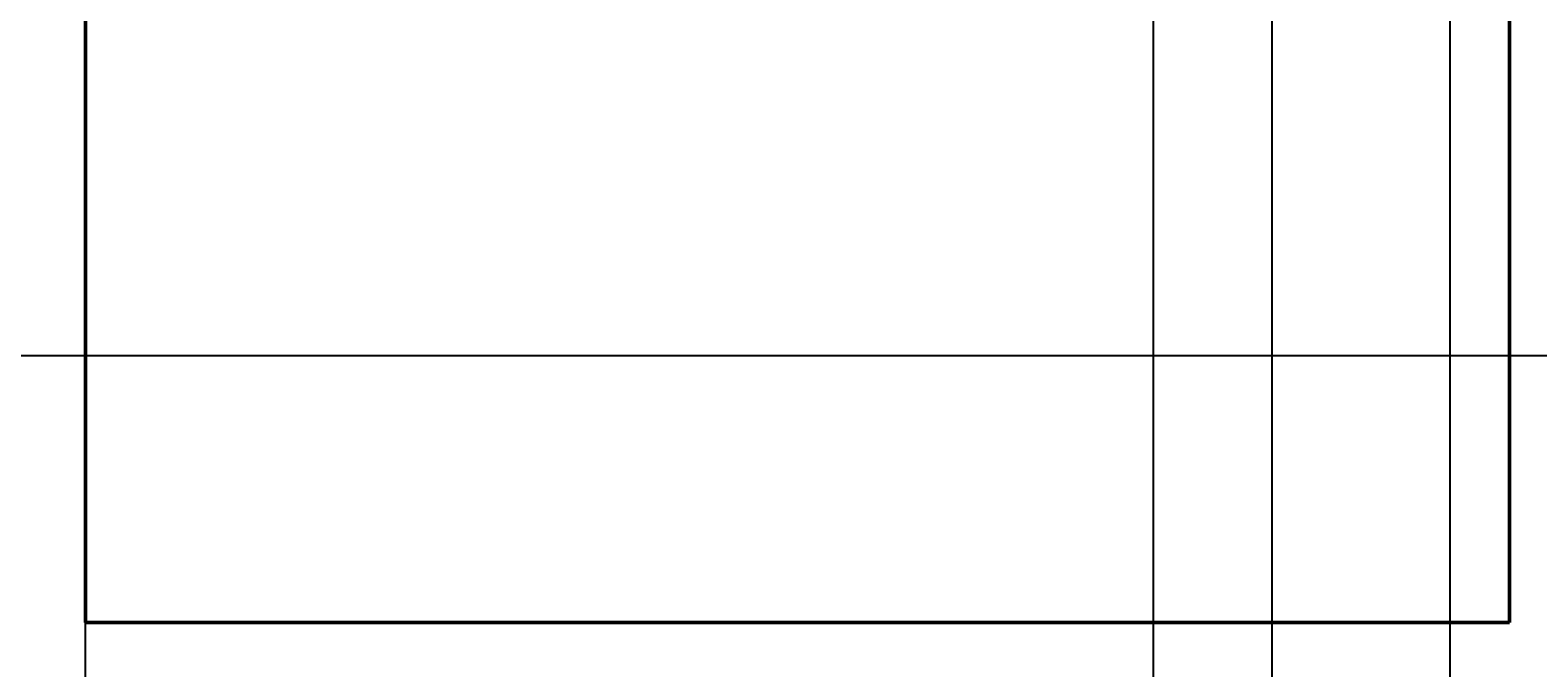
# Model space of a CAD drawing. Units: inches. Extents: x 37 to 824, y -700 to 234.
# Tile 44 of 77: x 168 to 219, y -4 to 17. Entities that reach past the tile are written whole.
import ezdxf

# ---------------------------------------------------------------- set-up
doc = ezdxf.new("R2010")
doc.units = ezdxf.units.IN
doc.header["$MEASUREMENT"] = 0
doc.layers.add('A-ANNO-DIMS', color=2, linetype='Continuous', lineweight=18)
doc.layers.add('A-WALL', color=2, linetype='Continuous', lineweight=50)
doc.styles.get("Standard").update_dxf_attribs({"font": 'arial.ttf'})
doc.dimstyles.get("Standard").update_dxf_attribs({"dimtxt": 0.18, "dimasz": 0.18, "dimexe": 0.18, "dimexo": 0.0625, "dimgap": 0.09, "dimtad": 0, "dimtih": 1, "dimtoh": 1, "dimdec": 1, "dimzin": 0, "dimdsep": 46, "dimlunit": 4, "dimtxsty": 'Standard', "dimcen": 0.09, "dimadec": 0, "dimazin": 0, "dimtfac": 1, "dimtdec": 1, "dimtofl": 0, "dimtmove": 0, "dimatfit": 3, "dimfxl": 1, "dimtolj": 1, "dimtzin": 0, "dimarcsym": 0})

# ---------------------------------------------------------------- blocks, each defined once
blk = doc.blocks.new('*D62')
at = {"layer": 'A-ANNO-DIMS', "color": 0, "lineweight": -2, "ltscale": 0.5, "transparency": 16777216}
for p, q in [((419.015, 6.09), (78.159, 6.09)), ((78.339, 5.91), (78.339, -10.728)), ((78.339, -27.73), (78.339, -11.091)), ((419.015, -27.91), (78.159, -27.91))]:
    blk.add_line(p, q, dxfattribs=at)
at = {"layer": 'A-ANNO-DIMS', "color": 0, "ltscale": 0.5, "transparency": 16777216}
for points in [[(78.309, 5.91), (78.369, 5.91), (78.339, 6.09)], [(78.309, -27.73), (78.369, -27.73), (78.339, -27.91)]]:
    blk.add_solid(points, dxfattribs=at)
at = {"layer": 'Defpoints', "color": 0, "ltscale": 0.5, "transparency": 16777216}
for p in [(419.077, 6.09), (78.339, -27.91), (419.077, -27.91)]:
    blk.add_point(p, dxfattribs=at)
at = {"layer": 'A-ANNO-DIMS', "color": 0, "ltscale": 0.5, "transparency": 16777216, "insert": (78.339, -10.91), "char_height": 0.18, "attachment_point": 5}
blk.add_mtext('\\A1;2\'-10"', dxfattribs=at)
blk = doc.blocks.new('*D84')
at = {"layer": 'A-ANNO-DIMS', "color": 0, "lineweight": -2, "ltscale": 0.5, "transparency": 16777216}
for p, q in [((170.077, -265.847), (170.077, 234.17)), ((170.257, 233.99), (189.748, 233.99)), ((209.897, 233.99), (190.406, 233.99)), ((210.077, -265.847), (210.077, 234.17))]:
    blk.add_line(p, q, dxfattribs=at)
at = {"layer": 'A-ANNO-DIMS', "color": 0, "ltscale": 0.5, "transparency": 16777216}
for points in [[(170.257, 234.02), (170.257, 233.96), (170.077, 233.99)], [(209.897, 234.02), (209.897, 233.96), (210.077, 233.99)]]:
    blk.add_solid(points, dxfattribs=at)
at = {"layer": 'Defpoints', "color": 0, "ltscale": 0.5, "transparency": 16777216}
for p in [(210.077, 233.99), (170.077, -265.91), (210.077, -265.91)]:
    blk.add_point(p, dxfattribs=at)
at = {"layer": 'A-ANNO-DIMS', "color": 0, "ltscale": 0.5, "transparency": 16777216, "insert": (190.077, 233.99), "char_height": 0.18, "attachment_point": 5}
blk.add_mtext('\\A1;3\'-4"', dxfattribs=at)
blk = doc.blocks.new('*D85')
at = {"layer": 'A-ANNO-DIMS', "color": 0, "lineweight": -2, "ltscale": 0.5, "transparency": 16777216}
for p, q in [((170.077, -356.847), (170.077, 234.17)), ((170.257, 233.99), (187.748, 233.99)), ((205.897, 233.99), (188.406, 233.99)), ((206.077, -356.847), (206.077, 234.17))]:
    blk.add_line(p, q, dxfattribs=at)
at = {"layer": 'A-ANNO-DIMS', "color": 0, "ltscale": 0.5, "transparency": 16777216}
for points in [[(170.257, 234.02), (170.257, 233.96), (170.077, 233.99)], [(205.897, 234.02), (205.897, 233.96), (206.077, 233.99)]]:
    blk.add_solid(points, dxfattribs=at)
at = {"layer": 'Defpoints', "color": 0, "ltscale": 0.5, "transparency": 16777216}
for p in [(206.077, 233.99), (170.077, -356.91), (206.077, -356.91)]:
    blk.add_point(p, dxfattribs=at)
at = {"layer": 'A-ANNO-DIMS', "color": 0, "ltscale": 0.5, "transparency": 16777216, "insert": (188.077, 233.99), "char_height": 0.18, "attachment_point": 5}
blk.add_mtext('\\A1;3\'-0"', dxfattribs=at)
blk = doc.blocks.new('*D86')
at = {"layer": 'A-ANNO-DIMS', "color": 0, "lineweight": -2, "ltscale": 0.5, "transparency": 16777216}
for p, q in [((206.077, -356.847), (206.077, 234.17)), ((206.257, 233.99), (210.678, 233.99)), ((215.897, 233.99), (211.476, 233.99)), ((216.077, -356.847), (216.077, 234.17))]:
    blk.add_line(p, q, dxfattribs=at)
at = {"layer": 'A-ANNO-DIMS', "color": 0, "ltscale": 0.5, "transparency": 16777216}
for points in [[(206.257, 234.02), (206.257, 233.96), (206.077, 233.99)], [(215.897, 234.02), (215.897, 233.96), (216.077, 233.99)]]:
    blk.add_solid(points, dxfattribs=at)
at = {"layer": 'Defpoints', "color": 0, "ltscale": 0.5, "transparency": 16777216}
for p in [(216.077, 233.99), (206.077, -356.91), (216.077, -356.91)]:
    blk.add_point(p, dxfattribs=at)
at = {"layer": 'A-ANNO-DIMS', "color": 0, "ltscale": 0.5, "transparency": 16777216, "insert": (211.077, 233.99), "char_height": 0.18, "attachment_point": 5}
blk.add_mtext('\\A1;0\'-10"', dxfattribs=at)
blk = doc.blocks.new('*D87')
at = {"layer": 'A-ANNO-DIMS', "color": 0, "lineweight": -2, "ltscale": 0.5, "transparency": 16777216}
for p, q in [((216.077, -356.847), (216.077, 234.17)), ((216.257, 233.99), (255.747, 233.99)), ((295.897, 233.99), (256.407, 233.99)), ((296.077, -356.847), (296.077, 234.17))]:
    blk.add_line(p, q, dxfattribs=at)
at = {"layer": 'A-ANNO-DIMS', "color": 0, "ltscale": 0.5, "transparency": 16777216}
for points in [[(216.257, 234.02), (216.257, 233.96), (216.077, 233.99)], [(295.897, 234.02), (295.897, 233.96), (296.077, 233.99)]]:
    blk.add_solid(points, dxfattribs=at)
at = {"layer": 'Defpoints', "color": 0, "ltscale": 0.5, "transparency": 16777216}
for p in [(296.077, 233.99), (216.077, -356.91), (296.077, -356.91)]:
    blk.add_point(p, dxfattribs=at)
at = {"layer": 'A-ANNO-DIMS', "color": 0, "ltscale": 0.5, "transparency": 16777216, "insert": (256.077, 233.99), "char_height": 0.18, "attachment_point": 5}
blk.add_mtext('\\A1;6\'-8"', dxfattribs=at)

msp = doc.modelspace()

# ---------------------------------------------------------------- linework, layer by layer
at = {"layer": 'A-WALL'}
for p, q in [((170.077, 75.09), (170.077, -2.91)), ((218.077, -2.91), (218.077, 46)), ((170.077, -2.91), (218.077, -2.91))]:
    msp.add_line(p, q, dxfattribs=at)

# ---------------------------------------------------------------- dimensions: what is measured, and where the dimension line sits
at = {"layer": 'A-ANNO-DIMS', "ltscale": 0.5}
for base, p1, p2, picture, middle in [((210.077, 233.99), (170.077, -265.91), (210.077, -265.91), '*D84', (190.077, 233.99)), ((206.077, 233.99), (170.077, -356.91), (206.077, -356.91), '*D85', (188.077, 233.99)), ((216.077, 233.99), (206.077, -356.91), (216.077, -356.91), '*D86', (211.077, 233.99)), ((296.077, 233.99), (216.077, -356.91), (296.077, -356.91), '*D87', (256.077, 233.99))]:
    dim = msp.add_linear_dim(base=base, p1=p1, p2=p2, dimstyle='Standard', override={"dimdec": 1, "dimlfac": 1, "dimrnd": 0, "dimzin": 1, "dimdsep": 46, "dimlunit": 4, "dimfrac": 2}, dxfattribs=at)
    dim.commit()
    dim.dimension.update_dxf_attribs({"geometry": picture, "text_midpoint": middle})
dim = msp.add_linear_dim(base=(78.339, -27.91), p1=(419.077, 6.09), p2=(419.077, -27.91), angle=90, dimstyle='Standard', override={"dimdec": 1, "dimlfac": 1, "dimrnd": 0, "dimzin": 1, "dimdsep": 46, "dimlunit": 4, "dimfrac": 2}, dxfattribs=at)
dim.commit()
dim.dimension.update_dxf_attribs({"geometry": '*D62', "text_midpoint": (78.339, -10.91)})

doc.saveas('drawing.dxf')
